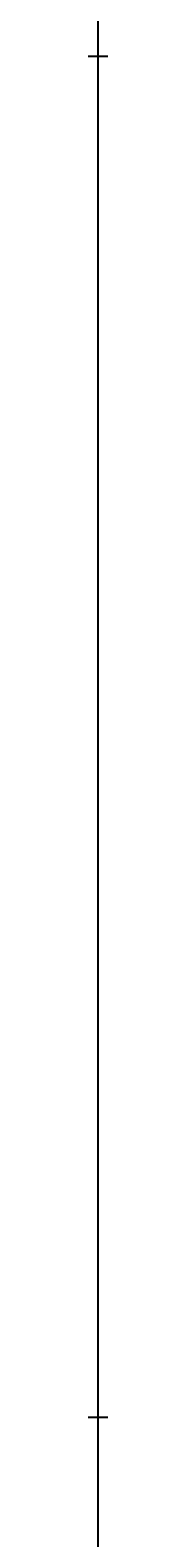
# Model space of a CAD drawing. Units: inches. Extents: x 35362 to 73946, y 43607 to 67532.
# Tile 37 of 134: x 48373 to 48373, y 46091 to 46564. Entities that reach past the tile are written whole.
import ezdxf

# ---------------------------------------------------------------- set-up
doc = ezdxf.new("R2010")
doc.units = ezdxf.units.IN
doc.header["$MEASUREMENT"] = 0
doc.layers.add('A-ANNO-DIMS', color=2, linetype='Continuous', lineweight=18)
doc.styles.get("Standard").update_dxf_attribs({"font": 'arial.ttf'})
doc.dimstyles.get("Standard").update_dxf_attribs({"dimtxt": 0.18, "dimasz": 0.18, "dimexe": 0.18, "dimexo": 0.0625, "dimgap": 0.09, "dimtad": 0, "dimtih": 1, "dimtoh": 1, "dimdec": 4, "dimzin": 0, "dimdsep": 46, "dimtxsty": 'Standard', "dimcen": 0.09, "dimadec": 0, "dimazin": 0, "dimtfac": 1, "dimtdec": 4, "dimtofl": 0, "dimtmove": 0, "dimatfit": 3, "dimfxl": 1, "dimtolj": 1, "dimtzin": 0, "dimarcsym": 0})

# ---------------------------------------------------------------- blocks, each defined once
blk = doc.blocks.new('*D5')
at = {"layer": 'A-ANNO-DIMS', "color": 0, "lineweight": -2, "transparency": 16777216}
for p, q in [((37121.95, 46919.32), (37121.95, 43606.68)), ((69871.5, 45449.83), (69871.5, 43606.68)), ((37122.13, 43606.86), (53496.29, 43606.86)), ((69871.32, 43606.86), (53497.15, 43606.86))]:
    blk.add_line(p, q, dxfattribs=at)
at = {"layer": 'A-ANNO-DIMS', "color": 0, "transparency": 16777216}
for points in [[(37122.13, 43606.89), (37122.13, 43606.83), (37121.95, 43606.86)], [(69871.32, 43606.89), (69871.32, 43606.83), (69871.5, 43606.86)]]:
    blk.add_solid(points, dxfattribs=at)
at = {"layer": 'Defpoints', "color": 0, "transparency": 16777216}
for p in [(37121.95, 46919.38), (69871.5, 45449.89), (69871.5, 43606.86)]:
    blk.add_point(p, dxfattribs=at)
at = {"layer": 'A-ANNO-DIMS', "color": 0, "transparency": 16777216, "insert": (53496.72, 43606.86), "char_height": 0.18, "attachment_point": 5}
blk.add_mtext('\\A1;32750', dxfattribs=at)
blk = doc.blocks.new('*D11')
at = {"layer": 'A-ANNO-DIMS', "color": 0, "lineweight": -2, "transparency": 16777216}
for p, q in [((47978.66, 56028.77), (47978.66, 43606.68)), ((53109.76, 56028.77), (53109.76, 43606.68)), ((47978.84, 43606.86), (50543.87, 43606.86)), ((53109.58, 43606.86), (50544.55, 43606.86))]:
    blk.add_line(p, q, dxfattribs=at)
at = {"layer": 'A-ANNO-DIMS', "color": 0, "transparency": 16777216}
for points in [[(47978.84, 43606.89), (47978.84, 43606.83), (47978.66, 43606.86)], [(53109.58, 43606.89), (53109.58, 43606.83), (53109.76, 43606.86)]]:
    blk.add_solid(points, dxfattribs=at)
at = {"layer": 'Defpoints', "color": 0, "transparency": 16777216}
for p in [(47978.66, 56028.84), (53109.76, 56028.84), (53109.76, 43606.86)]:
    blk.add_point(p, dxfattribs=at)
at = {"layer": 'A-ANNO-DIMS', "color": 0, "transparency": 16777216, "insert": (50544.21, 43606.86), "char_height": 0.18, "attachment_point": 5}
blk.add_mtext('\\A1;5131', dxfattribs=at)
blk = doc.blocks.new('*D13')
at = {"layer": 'A-ANNO-DIMS', "color": 0, "lineweight": -2, "transparency": 16777216}
for p, q in [((48373.49, 51694.02), (48373.49, 43606.68)), ((51029.04, 51694.02), (51029.04, 43606.68)), ((48373.67, 43606.86), (49700.8, 43606.86)), ((51028.86, 43606.86), (49701.73, 43606.86))]:
    blk.add_line(p, q, dxfattribs=at)
at = {"layer": 'A-ANNO-DIMS', "color": 0, "transparency": 16777216}
for points in [[(48373.67, 43606.89), (48373.67, 43606.83), (48373.49, 43606.86)], [(51028.86, 43606.89), (51028.86, 43606.83), (51029.04, 43606.86)]]:
    blk.add_solid(points, dxfattribs=at)
at = {"layer": 'Defpoints', "color": 0, "transparency": 16777216}
for p in [(48373.49, 51694.09), (51029.04, 51694.09), (51029.04, 43606.86)]:
    blk.add_point(p, dxfattribs=at)
at = {"layer": 'A-ANNO-DIMS', "color": 0, "transparency": 16777216, "insert": (49701.27, 43606.86), "char_height": 0.18, "attachment_point": 5}
blk.add_mtext('\\A1;2655.6', dxfattribs=at)
blk = doc.blocks.new('*D67')
at = {"layer": 'A-ANNO-DIMS', "color": 0, "lineweight": -2, "transparency": 16777216}
for p, q in [((56873.54, 53351.53), (35361.77, 53351.53)), ((35361.95, 53351.35), (35361.95, 49400.89)), ((35361.95, 45450.07), (35361.95, 49400.53)), ((53793.58, 45449.89), (35361.77, 45449.89))]:
    blk.add_line(p, q, dxfattribs=at)
at = {"layer": 'A-ANNO-DIMS', "color": 0, "transparency": 16777216}
for points in [[(35361.92, 53351.35), (35361.98, 53351.35), (35361.95, 53351.53)], [(35361.92, 45450.07), (35361.98, 45450.07), (35361.95, 45449.89)]]:
    blk.add_solid(points, dxfattribs=at)
at = {"layer": 'Defpoints', "color": 0, "transparency": 16777216}
for p in [(35361.95, 53351.53), (56873.6, 53351.53), (53793.64, 45449.89)]:
    blk.add_point(p, dxfattribs=at)
at = {"layer": 'A-ANNO-DIMS', "color": 0, "transparency": 16777216, "insert": (35361.95, 49400.71), "char_height": 0.18, "attachment_point": 5}
blk.add_mtext('\\A1;7901.6', dxfattribs=at)
blk = doc.blocks.new('*D76')
at = {"layer": 'A-ANNO-DIMS', "color": 0, "lineweight": -2, "transparency": 16777216}
for p, q in [((54052.84, 46555.29), (35361.77, 46555.29)), ((35361.95, 46555.11), (35361.95, 46342.27)), ((35361.95, 46129.06), (35361.95, 46341.9)), ((53793.58, 46128.88), (35361.77, 46128.88))]:
    blk.add_line(p, q, dxfattribs=at)
at = {"layer": 'A-ANNO-DIMS', "color": 0, "transparency": 16777216}
for points in [[(35361.92, 46555.11), (35361.98, 46555.11), (35361.95, 46555.29)], [(35361.92, 46129.06), (35361.98, 46129.06), (35361.95, 46128.88)]]:
    blk.add_solid(points, dxfattribs=at)
at = {"layer": 'Defpoints', "color": 0, "transparency": 16777216}
for p in [(35361.95, 46555.29), (54052.9, 46555.29), (53793.64, 46128.88)]:
    blk.add_point(p, dxfattribs=at)
at = {"layer": 'A-ANNO-DIMS', "color": 0, "transparency": 16777216, "insert": (35361.95, 46342.09), "char_height": 0.18, "attachment_point": 5}
blk.add_mtext('\\A1;426.4', dxfattribs=at)
blk = doc.blocks.new('*D90')
at = {"layer": 'A-ANNO-DIMS', "color": 0, "lineweight": -2, "transparency": 16777216}
for p, q in [((53707.72, 47291.29), (35361.77, 47291.29)), ((35361.95, 47291.11), (35361.95, 46710.26)), ((35361.95, 46129.06), (35361.95, 46709.9)), ((53793.58, 46128.88), (35361.77, 46128.88))]:
    blk.add_line(p, q, dxfattribs=at)
at = {"layer": 'A-ANNO-DIMS', "color": 0, "transparency": 16777216}
for points in [[(35361.92, 47291.11), (35361.98, 47291.11), (35361.95, 47291.29)], [(35361.92, 46129.06), (35361.98, 46129.06), (35361.95, 46128.88)]]:
    blk.add_solid(points, dxfattribs=at)
at = {"layer": 'Defpoints', "color": 0, "transparency": 16777216}
for p in [(53707.78, 47291.29), (35361.95, 46128.88), (53793.64, 46128.88)]:
    blk.add_point(p, dxfattribs=at)
at = {"layer": 'A-ANNO-DIMS', "color": 0, "transparency": 16777216, "insert": (35361.95, 46710.08), "char_height": 0.18, "attachment_point": 5}
blk.add_mtext('\\A1;1162.4', dxfattribs=at)

msp = doc.modelspace()

# ---------------------------------------------------------------- dimensions: what is measured, and where the dimension line sits
at = {"layer": 'A-ANNO-DIMS'}
for base, p1, p2, override, picture, middle in [((53109.76, 43606.859), (47978.665, 56028.836), (53109.76, 56028.836), {"dimdec": 0, "dimlfac": 1, "dimrnd": 0, "dimzin": 0, "dimdsep": 46, "dimlunit": 2}, '*D11', (50544.212, 43606.859)), ((51029.043, 43606.859), (48373.492, 51694.087), (51029.043, 51694.087), {"dimdec": 1, "dimlfac": 1, "dimrnd": 0, "dimzin": 0, "dimdsep": 46, "dimlunit": 2}, '*D13', (49701.267, 43606.859)), ((69871.496, 43606.859), (37121.949, 46919.381), (69871.496, 45449.894), {"dimdec": 0, "dimlfac": 1, "dimrnd": 0, "dimzin": 0, "dimdsep": 46, "dimlunit": 2}, '*D5', (53496.723, 43606.859))]:
    dim = msp.add_linear_dim(base=base, p1=p1, p2=p2, dimstyle='Standard', override=override, dxfattribs=at)
    dim.commit()
    dim.dimension.update_dxf_attribs({"geometry": picture, "text_midpoint": middle})
for base, p1, p2, picture, middle in [((35361.949, 53351.529), (53793.638, 45449.894), (56873.602, 53351.529), '*D67', (35361.949, 49400.712)), ((35361.949, 46128.878), (53707.781, 47291.285), (53793.638, 46128.878), '*D90', (35361.949, 46710.081)), ((35361.949, 46555.293), (53793.638, 46128.878), (54052.899, 46555.293), '*D76', (35361.949, 46342.086))]:
    dim = msp.add_linear_dim(base=base, p1=p1, p2=p2, angle=90, dimstyle='Standard', override={"dimdec": 1, "dimlfac": 1, "dimrnd": 0, "dimzin": 0, "dimdsep": 46, "dimlunit": 2}, dxfattribs=at)
    dim.commit()
    dim.dimension.update_dxf_attribs({"geometry": picture, "text_midpoint": middle})

doc.saveas('drawing.dxf')
